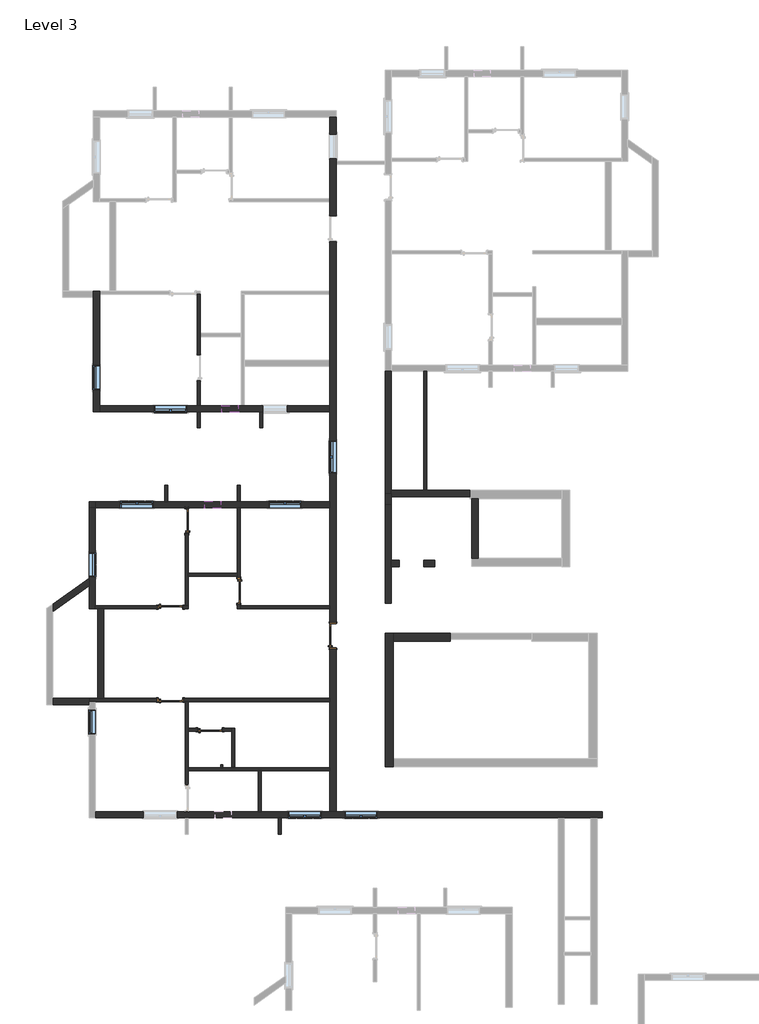
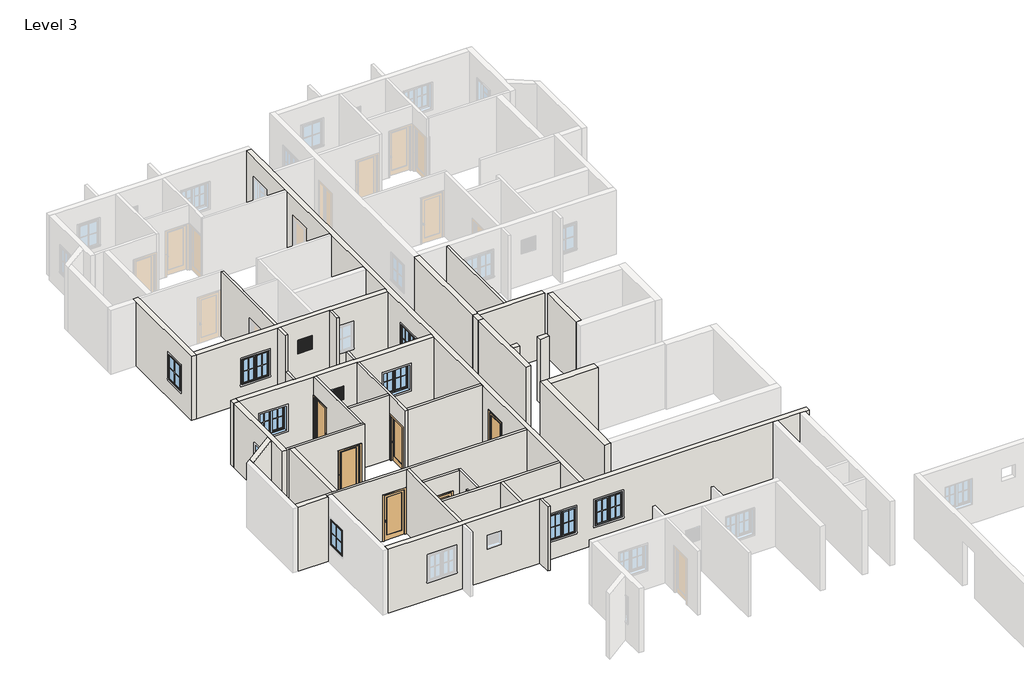
# One storey, part 4 of 7: 38 walls, 11 windows, 6 doors.
"""IFC4 building model written with IfcOpenShell, lengths in millimetres."""

from ifc_helpers import new_model, si_unit, frame, origin, place, context, project, spatial, polyline, outline, extrude, faceted_brep, transform, mapped, element, save
from components import door_a3feeac7, door_3c6ab76a, door_3b97b8e7, window_272f20d6, window_casement_double_4_x_4_af3140d2, window_f2d8fef0

model = new_model("IFC4")

# Units and contexts
model_context = context("Model", 3, world=origin())
ifc_project = project(units=[si_unit("LENGTHUNIT", "METRE", prefix="MILLI")], contexts=[model_context])

# Site, building, storey
site = spatial("IfcSite", under=ifc_project)
building = spatial("IfcBuilding", under=site)
storey = spatial("IfcBuildingStorey", under=building, Name="Level 3", Elevation=3200.4)

# Doors
placement = place(None, origin())
door_shape = door_a3feeac7(model_context)
element("IfcDoor", 1, ObjectType="Door-Interior-Single-1_Panel-Wood : 2'6\" x 7' door", at=placement, inside=storey, context=model_context, shape_type="MappedRepresentation", body=[
    mapped(door_shape, transform((-11252.4759469, 12427.2461172, 3200.4), x_axis=(0.0, 1.0, 0.0), y_axis=(-1.0, 0.0, 0.0), z_axis=(0.0, 0.0, 1.0))),
])
element("IfcDoor", 2, ObjectType="Door-Interior-Single-1_Panel-Wood : 2'6\" x 7' door", at=placement, inside=storey, context=model_context, shape_type="MappedRepresentation", body=[
    mapped(door_shape, transform((-10385.7009469, 4632.6211172, 3200.4), x_axis=(1.0, 0.0, 0.0), y_axis=(0.0, 1.0, 0.0), z_axis=(0.0, 0.0, 1.0))),
])
door_2_shape = door_3c6ab76a(model_context)
element("IfcDoor", 3, ObjectType="Door-Interior-Single-1_Panel-Wood : 36\" x 84\"", at=placement, inside=storey, context=model_context, shape_type="MappedRepresentation", body=[
    mapped(door_2_shape, transform((-9309.3759469, 9817.3961172, 3200.4), x_axis=(0.0, -1.0, 0.0), y_axis=(1.0, 0.0, 0.0), z_axis=(0.0, 0.0, 1.0))),
])
element("IfcDoor", 4, ObjectType="Door-Interior-Single-1_Panel-Wood : 36\" x 84\"", at=placement, inside=storey, context=model_context, shape_type="MappedRepresentation", body=[
    mapped(door_2_shape, transform((-11865.2509469, 9210.9711172, 3200.4), x_axis=(1.0, 0.0, 0.0), y_axis=(0.0, 1.0, 0.0), z_axis=(0.0, 0.0, 1.0))),
])
door_3_shape = door_3b97b8e7(model_context)
element("IfcDoor", 5, ObjectType="Door-Interior-Single-1_Panel-Wood : 36\" x 84\"", at=placement, inside=storey, context=model_context, shape_type="MappedRepresentation", body=[
    mapped(door_3_shape, transform((-5791.4759469, 8140.9961172, 3200.4), x_axis=(0.0, 1.0, 0.0), y_axis=(-1.0, 0.0, 0.0), z_axis=(0.0, 0.0, 1.0))),
])
element("IfcDoor", 6, ObjectType="Door-Interior-Single-1_Panel-Wood : 36\" x 84\"", at=placement, inside=storey, context=model_context, shape_type="MappedRepresentation", body=[
    mapped(door_shape, transform((-11865.2509469, 5737.5211172, 3200.4), x_axis=(1.0, 0.0, 0.0), y_axis=(0.0, 1.0, 0.0), z_axis=(0.0, 0.0, 1.0))),
])

# Walls
element("IfcWall", 7, ObjectType="1' feet", at=placement, inside=storey, context=model_context, shape_type="Brep", body=[
    faceted_brep([(-3540.4009469, 3245.1461172, 3200.4), (-3540.4009469, 3549.9461172, 3200.4), (-3540.4009469, 7931.4461172, 3200.4), (-3540.4009469, 8236.2461172, 3200.4), (-3540.4009469, 8236.2461172, 6248.4), (-3540.4009469, 7931.4461172, 6248.4), (-3540.4009469, 3549.9461172, 6248.4), (-3540.4009469, 3245.1461172, 6248.4), (-3845.2009469, 3245.1461172, 3200.4), (-3845.2009469, 3245.1461172, 6248.4), (-3845.2009469, 8236.2461172, 6248.4), (-3845.2009469, 8236.2461172, 3200.4)], [[[0, 1, 2, 3, 4, 5, 6, 7]], [[8, 9, 10, 11]], [[3, 2, 1, 0, 8, 11]], [[7, 6, 5, 4, 10, 9]], [[4, 3, 11, 10]], [[0, 7, 9, 8]]]),
])
element("IfcWall", 8, ObjectType="1' feet", at=placement, inside=storey, context=model_context, shape_type="Brep", body=[
    faceted_brep([(-3540.4009469, 7931.4461172, 3200.4), (-1406.8009469, 7931.4461172, 3200.4), (-1406.8009469, 7931.4461172, 6248.4), (-3540.4009469, 7931.4461172, 6248.4), (-3540.4009469, 8236.2461172, 3200.4), (-3540.4009469, 8236.2461172, 6248.4), (-1406.8009469, 8236.2461172, 6248.4), (-1406.8009469, 8236.2461172, 3200.4), (-1406.8009469, 8007.6461172, 3200.4), (-1406.8009469, 8007.6461172, 6248.4)], [[[0, 1, 2, 3]], [[4, 5, 6, 7]], [[1, 0, 4, 7, 8]], [[2, 1, 8, 7, 6, 9]], [[3, 2, 9, 6, 5]], [[0, 3, 5, 4]]]),
])
element("IfcWall", 9, ObjectType="4.5\" wall", at=placement, inside=storey, context=model_context, shape_type="Brep", body=[
    faceted_brep([(-10741.3009469, 20898.1461172, 6248.4), (-10741.3009469, 19437.6461172, 6248.4), (-10741.3009469, 19323.3461172, 6248.4), (-10741.3009469, 16732.5461172, 6248.4), (-10741.3009469, 16732.5461172, 3200.4), (-10741.3009469, 17678.6961172, 3200.4), (-10741.3009469, 17678.6961172, 5359.4), (-10741.3009469, 18643.8961172, 5359.4), (-10741.3009469, 18643.8961172, 3200.4), (-10741.3009469, 19323.3461172, 3200.4), (-10741.3009469, 19437.6461172, 3200.4), (-10741.3009469, 20898.1461172, 3200.4), (-10855.6009469, 16732.5461172, 6248.4), (-10855.6009469, 20898.1461172, 6248.4), (-10855.6009469, 20898.1461172, 3200.4), (-10855.6009469, 18643.8961172, 3200.4), (-10855.6009469, 18643.8961172, 5359.4), (-10855.6009469, 17678.6961172, 5359.4), (-10855.6009469, 17678.6961172, 3200.4), (-10855.6009469, 16732.5461172, 3200.4)], [[[0, 1, 2, 3, 4, 5, 6, 7, 8, 9, 10, 11]], [[12, 13, 14, 15, 16, 17, 18, 19]], [[4, 19, 18, 5]], [[14, 11, 10, 9, 8, 15]], [[3, 2, 1, 0, 13, 12]], [[4, 3, 12, 19]], [[0, 11, 14, 13]], [[7, 16, 15, 8]], [[16, 7, 6, 17]], [[17, 6, 5, 18]]]),
])
element("IfcWall", 10, ObjectType="4.5\" wall", at=placement, inside=storey, context=model_context, shape_type="Brep", body=[
    faceted_brep([(-9369.7009469, 9150.6461172, 6248.4), (-9369.7009469, 10369.8461172, 6248.4), (-9369.7009469, 10484.1461172, 6248.4), (-9369.7009469, 12922.5461172, 6248.4), (-9369.7009469, 12922.5461172, 3200.4), (-9369.7009469, 10484.1461172, 3200.4), (-9369.7009469, 10369.8461172, 3200.4), (-9369.7009469, 10299.9961172, 3200.4), (-9369.7009469, 10299.9961172, 5359.4), (-9369.7009469, 9334.7961172, 5359.4), (-9369.7009469, 9334.7961172, 3200.4), (-9369.7009469, 9150.6461172, 3200.4), (-9255.4009469, 12922.5461172, 6248.4), (-9255.4009469, 9264.9461172, 6248.4), (-9255.4009469, 9150.6461172, 6248.4), (-9255.4009469, 9150.6461172, 3200.4), (-9255.4009469, 9264.9461172, 3200.4), (-9255.4009469, 9334.7961172, 3200.4), (-9255.4009469, 9334.7961172, 5359.4), (-9255.4009469, 10299.9961172, 5359.4), (-9255.4009469, 10299.9961172, 3200.4), (-9255.4009469, 12922.5461172, 3200.4)], [[[0, 1, 2, 3, 4, 5, 6, 7, 8, 9, 10, 11]], [[12, 13, 14, 15, 16, 17, 18, 19, 20, 21]], [[4, 21, 20, 7, 6, 5]], [[15, 11, 10, 17, 16]], [[3, 2, 1, 0, 14, 13, 12]], [[4, 3, 12, 21]], [[0, 11, 15, 14]], [[9, 18, 17, 10]], [[18, 9, 8, 19]], [[19, 8, 7, 20]]]),
])
element("IfcWall", 11, ObjectType="4.5\" wall", at=placement, inside=storey, context=model_context, shape_type="SweptSolid", body=[
    extrude(outline(polyline([(-11198.5009469, 10484.1461172), (-9369.7009469, 10484.1461172), (-9369.7009469, 10369.8461172), (-11198.5009469, 10369.8461172), (-11198.5009469, 10484.1461172)])), frame((0.0, 0.0, 3200.4), z_axis=(0.0, 0.0, 1.0), x_axis=(1.0, 0.0, 0.0)), (0.0, 0.0, 1.0), 3048.0),
])
element("IfcWall", 12, ObjectType="4.5\" wall", at=placement, inside=storey, context=model_context, shape_type="Brep", body=[
    faceted_brep([(-11312.8009469, 9264.9461172, 6248.4), (-11312.8009469, 12922.5461172, 6248.4), (-11312.8009469, 12922.5461172, 3200.4), (-11312.8009469, 12909.8461172, 3200.4), (-11312.8009469, 12909.8461172, 5359.4), (-11312.8009469, 11944.6461172, 5359.4), (-11312.8009469, 11944.6461172, 3200.4), (-11312.8009469, 9264.9461172, 3200.4), (-11198.5009469, 12922.5461172, 6248.4), (-11198.5009469, 10484.1461172, 6248.4), (-11198.5009469, 10369.8461172, 6248.4), (-11198.5009469, 9264.9461172, 6248.4), (-11198.5009469, 9264.9461172, 3200.4), (-11198.5009469, 10369.8461172, 3200.4), (-11198.5009469, 10484.1461172, 3200.4), (-11198.5009469, 11944.6461172, 3200.4), (-11198.5009469, 11944.6461172, 5359.4), (-11198.5009469, 12909.8461172, 5359.4), (-11198.5009469, 12909.8461172, 3200.4), (-11198.5009469, 12922.5461172, 3200.4)], [[[0, 1, 2, 3, 4, 5, 6, 7]], [[8, 9, 10, 11, 12, 13, 14, 15, 16, 17, 18, 19]], [[12, 7, 6, 15, 14, 13]], [[2, 19, 18, 3]], [[1, 0, 11, 10, 9, 8]], [[0, 7, 12, 11]], [[2, 1, 8, 19]], [[17, 4, 3, 18]], [[4, 17, 16, 5]], [[5, 16, 15, 6]]]),
])
element("IfcWall", 13, ObjectType="4.5\" wall", at=placement, inside=storey, context=model_context, shape_type="Brep", body=[
    faceted_brep([(-14665.6009469, 9264.9461172, 6248.4), (-11312.8009469, 9264.9461172, 6248.4), (-11198.5009469, 9264.9461172, 6248.4), (-11198.5009469, 9264.9461172, 3200.4), (-11312.8009469, 9264.9461172, 3200.4), (-11382.6509469, 9264.9461172, 3200.4), (-11382.6509469, 9264.9461172, 5359.4), (-12347.8509469, 9264.9461172, 5359.4), (-12347.8509469, 9264.9461172, 3200.4), (-14665.6009469, 9264.9461172, 3200.4), (-11198.5009469, 9150.6461172, 6248.4), (-14360.8009469, 9150.6461172, 6248.4), (-14589.4009469, 9150.6461172, 6248.4), (-14665.6009469, 9150.6461172, 6248.4), (-14665.6009469, 9150.6461172, 3200.4), (-14589.4009469, 9150.6461172, 3200.4), (-14360.8009469, 9150.6461172, 3200.4), (-12347.8509469, 9150.6461172, 3200.4), (-12347.8509469, 9150.6461172, 5359.4), (-11382.6509469, 9150.6461172, 5359.4), (-11382.6509469, 9150.6461172, 3200.4), (-11198.5009469, 9150.6461172, 3200.4)], [[[0, 1, 2, 3, 4, 5, 6, 7, 8, 9]], [[10, 11, 12, 13, 14, 15, 16, 17, 18, 19, 20, 21]], [[3, 21, 20, 5, 4]], [[14, 9, 8, 17, 16, 15]], [[2, 1, 0, 13, 12, 11, 10]], [[3, 2, 10, 21]], [[0, 9, 14, 13]], [[19, 6, 5, 20]], [[6, 19, 18, 7]], [[7, 18, 17, 8]]]),
])
element("IfcWall", 14, ObjectType="4.5\" wall", at=placement, inside=storey, context=model_context, shape_type="SweptSolid", body=[
    extrude(outline(polyline([(-9255.4009469, 9264.9461172), (-5902.6009469, 9264.9461172), (-5902.6009469, 9150.6461172), (-9255.4009469, 9150.6461172), (-9255.4009469, 9264.9461172)])), frame((0.0, 0.0, 3200.4), z_axis=(0.0, 0.0, 1.0), x_axis=(1.0, 0.0, 0.0)), (0.0, 0.0, 1.0), 3048.0),
])
element("IfcWall", 15, ObjectType="4.5\" wall", at=placement, inside=storey, context=model_context, shape_type="Brep", body=[
    faceted_brep([(-5902.6009469, 5683.5461172, 6248.4), (-11198.5009469, 5683.5461172, 6248.4), (-11312.8009469, 5683.5461172, 6248.4), (-14665.6009469, 5683.5461172, 6248.4), (-14894.2009469, 5683.5461172, 6248.4), (-14894.2009469, 5683.5461172, 3200.4), (-14665.6009469, 5683.5461172, 3200.4), (-12347.8509469, 5683.5461172, 3200.4), (-12347.8509469, 5683.5461172, 5359.4), (-11382.6509469, 5683.5461172, 5359.4), (-11382.6509469, 5683.5461172, 3200.4), (-11312.8009469, 5683.5461172, 3200.4), (-11198.5009469, 5683.5461172, 3200.4), (-5902.6009469, 5683.5461172, 3200.4), (-14894.2009469, 5797.8461172, 6248.4), (-14589.4009469, 5797.8461172, 6248.4), (-14360.8009469, 5797.8461172, 6248.4), (-5902.6009469, 5797.8461172, 6248.4), (-5902.6009469, 5797.8461172, 3200.4), (-11382.6509469, 5797.8461172, 3200.4), (-11382.6509469, 5797.8461172, 5359.4), (-12347.8509469, 5797.8461172, 5359.4), (-12347.8509469, 5797.8461172, 3200.4), (-14360.8009469, 5797.8461172, 3200.4), (-14589.4009469, 5797.8461172, 3200.4), (-14894.2009469, 5797.8461172, 3200.4)], [[[0, 1, 2, 3, 4, 5, 6, 7, 8, 9, 10, 11, 12, 13]], [[14, 15, 16, 17, 18, 19, 20, 21, 22, 23, 24, 25]], [[18, 13, 12, 11, 10, 19]], [[5, 25, 24, 23, 22, 7, 6]], [[4, 3, 2, 1, 0, 17, 16, 15, 14]], [[0, 13, 18, 17]], [[5, 4, 14, 25]], [[9, 20, 19, 10]], [[20, 9, 8, 21]], [[21, 8, 7, 22]]]),
])
element("IfcWall", 16, ObjectType="4.5\" wall", at=placement, inside=storey, context=model_context, shape_type="Brep", body=[
    faceted_brep([(-11198.5009469, 5683.5461172, 6248.4), (-11198.5009469, 4692.9461172, 6248.4), (-11198.5009469, 4578.6461172, 6248.4), (-11198.5009469, 3207.0461172, 6248.4), (-11198.5009469, 3092.7461172, 6248.4), (-11198.5009469, 1568.7461172, 6248.4), (-11198.5009469, 1568.7461172, 3200.4), (-11198.5009469, 1581.4461172, 3200.4), (-11198.5009469, 1581.4461172, 5359.4), (-11198.5009469, 2546.6461172, 5359.4), (-11198.5009469, 2546.6461172, 3200.4), (-11198.5009469, 3092.7461172, 3200.4), (-11198.5009469, 3207.0461172, 3200.4), (-11198.5009469, 4578.6461172, 3200.4), (-11198.5009469, 4692.9461172, 3200.4), (-11198.5009469, 5683.5461172, 3200.4), (-11312.8009469, 1568.7461172, 6248.4), (-11312.8009469, 5683.5461172, 6248.4), (-11312.8009469, 5683.5461172, 3200.4), (-11312.8009469, 2546.6461172, 3200.4), (-11312.8009469, 2546.6461172, 5359.4), (-11312.8009469, 1581.4461172, 5359.4), (-11312.8009469, 1581.4461172, 3200.4), (-11312.8009469, 1568.7461172, 3200.4)], [[[0, 1, 2, 3, 4, 5, 6, 7, 8, 9, 10, 11, 12, 13, 14, 15]], [[16, 17, 18, 19, 20, 21, 22, 23]], [[18, 15, 14, 13, 12, 11, 10, 19]], [[6, 23, 22, 7]], [[5, 4, 3, 2, 1, 0, 17, 16]], [[0, 15, 18, 17]], [[6, 5, 16, 23]], [[21, 8, 7, 22]], [[8, 21, 20, 9]], [[9, 20, 19, 10]]]),
])
element("IfcWall", 17, ObjectType="4.5\" wall", at=placement, inside=storey, context=model_context, shape_type="SweptSolid", body=[
    extrude(outline(polyline([(-9985.226836, 3326.5226372), (-9915.376836, 3326.5226372), (-9915.376836, 3212.2226372), (-9985.226836, 3212.2226372), (-9985.226836, 3326.5226372)])), frame((0.0, 0.0, 3200.4), z_axis=(0.0, 0.0, 1.0), x_axis=(1.0, 0.0, 0.0)), (0.0, 0.0, 1.0), 3048.0),
])
element("IfcWall", 18, ObjectType="4.5\" wall", at=placement, inside=storey, context=model_context, shape_type="Brep", body=[
    faceted_brep([(-5902.6009469, 3207.0461172, 3200.4), (-11198.5009469, 3207.0461172, 3200.4), (-11198.5009469, 3207.0461172, 6248.4), (-5902.6009469, 3207.0461172, 6248.4), (-5902.6009469, 3092.7461172, 3200.4), (-5902.6009469, 3092.7461172, 6248.4), (-8468.0009469, 3092.7461172, 6248.4), (-8582.3009469, 3092.7461172, 6248.4), (-11198.5009469, 3092.7461172, 6248.4), (-11198.5009469, 3092.7461172, 3200.4), (-8582.3009469, 3092.7461172, 3200.4), (-8468.0009469, 3092.7461172, 3200.4)], [[[0, 1, 2, 3]], [[4, 5, 6, 7, 8, 9, 10, 11]], [[1, 0, 4, 11, 10, 9]], [[3, 2, 8, 7, 6, 5]], [[2, 1, 9, 8]], [[0, 3, 5, 4]]]),
])
element("IfcWall", 19, ObjectType="4.5\" wall", at=placement, inside=storey, context=model_context, shape_type="SweptSolid", body=[
    extrude(outline(polyline([(-8582.3009469, 1568.7461172), (-8582.3009469, 3092.7461172), (-8468.0009469, 3092.7461172), (-8468.0009469, 1568.7461172), (-8582.3009469, 1568.7461172)])), frame((0.0, 0.0, 3200.4), z_axis=(0.0, 0.0, 1.0), x_axis=(1.0, 0.0, 0.0)), (0.0, 0.0, 1.0), 3048.0),
])
element("IfcWall", 20, ObjectType="4.5\" wall", at=placement, inside=storey, context=model_context, shape_type="Brep", body=[
    faceted_brep([(-9572.9009469, 4692.9461172, 3200.4), (-9572.9009469, 4578.6461172, 3200.4), (-9572.9009469, 3245.1461172, 3200.4), (-9572.9009469, 3245.1461172, 6248.4), (-9572.9009469, 4578.6461172, 6248.4), (-9572.9009469, 4692.9461172, 6248.4), (-9458.6009469, 4692.9461172, 3200.4), (-9458.6009469, 4692.9461172, 6248.4), (-9458.6009469, 3245.1461172, 6248.4), (-9458.6009469, 3245.1461172, 3200.4)], [[[0, 1, 2, 3, 4, 5]], [[6, 7, 8, 9]], [[2, 1, 0, 6, 9]], [[3, 2, 9, 8]], [[5, 4, 3, 8, 7]], [[0, 5, 7, 6]]]),
])
element("IfcWall", 21, ObjectType="4.5\" wall", at=placement, inside=storey, context=model_context, shape_type="SweptSolid", body=[
    extrude(outline(polyline([(6248.4, -9572.9009469), (6248.4, -11198.5009469), (3200.4, -11198.5009469), (3200.4, -10868.3009469), (5359.4, -10868.3009469), (5359.4, -9903.1009469), (3200.4, -9903.1009469), (3200.4, -9572.9009469), (6248.4, -9572.9009469)])), frame((0.0, 4578.6461172, 0.0), z_axis=(0.0, 1.0, 0.0), x_axis=(0.0, 0.0, 1.0)), (0.0, 0.0, 1.0), 114.3),
])
element("IfcWall", 22, ObjectType="4.5\" wall", at=placement, inside=storey, context=model_context, shape_type="SweptSolid", body=[
    extrude(outline(polyline([(-7841.0333092, 730.5461172), (-7841.0333092, 1340.1461172), (-7726.7333092, 1340.1461172), (-7726.7333092, 730.5461172), (-7841.0333092, 730.5461172)])), frame((0.0, 0.0, 3200.4), z_axis=(0.0, 0.0, 1.0), x_axis=(1.0, 0.0, 0.0)), (0.0, 0.0, 1.0), 3048.0),
])
element("IfcWall", 23, ObjectType="4.5\" wall", at=placement, inside=storey, context=model_context, shape_type="SweptSolid", body=[
    extrude(outline(polyline([(-10855.6009469, 15918.3895495), (-10855.6009469, 16503.9461172), (-10741.3009469, 16503.9461172), (-10741.3009469, 15918.3895495), (-10855.6009469, 15918.3895495)])), frame((0.0, 0.0, 3200.4), z_axis=(0.0, 0.0, 1.0), x_axis=(1.0, 0.0, 0.0)), (0.0, 0.0, 1.0), 3048.0),
])
element("IfcWall", 24, ObjectType="4.5\" wall", at=placement, inside=storey, context=model_context, shape_type="Brep", body=[
    faceted_brep([(-8531.5009469, 16503.9461172, 3200.4), (-8531.5009469, 15918.3895495, 3200.4), (-8531.5009469, 15918.3895495, 6248.4), (-8531.5009469, 16503.9461172, 6248.4), (-8417.2009469, 16503.9461172, 3200.4), (-8417.2009469, 16503.9461172, 4114.8), (-8417.2009469, 16503.9461172, 5334.0), (-8417.2009469, 16503.9461172, 6248.4), (-8417.2009469, 15918.3895495, 6248.4), (-8417.2009469, 15918.3895495, 3200.4)], [[[0, 1, 2, 3]], [[4, 5, 6, 7, 8, 9]], [[1, 0, 4, 9]], [[2, 1, 9, 8]], [[3, 2, 8, 7]], [[0, 3, 7, 6, 5, 4]]]),
])
element("IfcWall", 25, ObjectType="4.5\" wall", at=placement, inside=storey, context=model_context, shape_type="SweptSolid", body=[
    extrude(outline(polyline([(-12085.9698258, 13151.1461172), (-12085.9698258, 13760.7461172), (-11971.6698258, 13760.7461172), (-11971.6698258, 13151.1461172), (-12085.9698258, 13151.1461172)])), frame((0.0, 0.0, 3200.4), z_axis=(0.0, 0.0, 1.0), x_axis=(1.0, 0.0, 0.0)), (0.0, 0.0, 1.0), 3048.0),
])
element("IfcWall", 26, ObjectType="4.5\" wall", at=placement, inside=storey, context=model_context, shape_type="SweptSolid", body=[
    extrude(outline(polyline([(-9255.4009469, 13760.7461172), (-9255.4009469, 13151.1461172), (-9369.7009469, 13151.1461172), (-9369.7009469, 13760.7461172), (-9255.4009469, 13760.7461172)])), frame((0.0, 0.0, 3200.4), z_axis=(0.0, 0.0, 1.0), x_axis=(1.0, 0.0, 0.0)), (0.0, 0.0, 1.0), 3048.0),
])
element("IfcWall", 27, ObjectType="4.5\" wall", at=placement, inside=storey, context=model_context, shape_type="SweptSolid", body=[
    extrude(outline(polyline([(-2402.381873, 13571.4182723), (-2402.381873, 18017.4255084), (-2288.081873, 18017.4255084), (-2288.081873, 13571.4182723), (-2402.381873, 13571.4182723)])), frame((0.0, 0.0, 3200.4), z_axis=(0.0, 0.0, 1.0), x_axis=(1.0, 0.0, 0.0)), (0.0, 0.0, 1.0), 3048.0),
])
element("IfcWall", 28, ObjectType="9\"", at=placement, inside=storey, context=model_context, shape_type="Brep", body=[
    faceted_brep([(-14513.2009469, 16503.9461172, 3200.4), (-14513.2009469, 16732.5461172, 3200.4), (-14513.2009469, 20898.1461172, 3200.4), (-14513.2009469, 21012.4461172, 3200.4), (-14513.2009469, 21012.4461172, 6248.4), (-14513.2009469, 20898.1461172, 6248.4), (-14513.2009469, 16732.5461172, 6248.4), (-14513.2009469, 16503.9461172, 6248.4), (-14513.2009469, 18243.8461172, 5334.0), (-14513.2009469, 18243.8461172, 4114.8), (-14513.2009469, 17329.4461172, 4114.8), (-14513.2009469, 17329.4461172, 5334.0), (-14741.8009469, 16503.9461172, 3200.4), (-14741.8009469, 16503.9461172, 6248.4), (-14741.8009469, 20783.8461172, 6248.4), (-14741.8009469, 21012.4461172, 6248.4), (-14741.8009469, 21012.4461172, 3200.4), (-14741.8009469, 20783.8461172, 3200.4), (-14741.8009469, 18243.8461172, 5334.0), (-14741.8009469, 17329.4461172, 5334.0), (-14741.8009469, 17329.4461172, 4114.8), (-14741.8009469, 18243.8461172, 4114.8)], [[[0, 1, 2, 3, 4, 5, 6, 7], [8, 9, 10, 11]], [[12, 13, 14, 15, 16, 17], [18, 19, 20, 21]], [[3, 2, 1, 0, 12, 17, 16]], [[7, 6, 5, 4, 15, 14, 13]], [[4, 3, 16, 15]], [[0, 7, 13, 12]], [[9, 8, 18, 21]], [[10, 9, 21, 20]], [[11, 10, 20, 19]], [[8, 11, 19, 18]]]),
])
element("IfcWall", 29, ObjectType="9\"", at=placement, inside=storey, context=model_context, shape_type="Brep", body=[
    faceted_brep([(-5902.6009469, 1568.7461172, 6248.4), (-5902.6009469, 3092.7461172, 6248.4), (-5902.6009469, 3207.0461172, 6248.4), (-5902.6009469, 5683.5461172, 6248.4), (-5902.6009469, 5797.8461172, 6248.4), (-5902.6009469, 9150.6461172, 6248.4), (-5902.6009469, 9264.9461172, 6248.4), (-5902.6009469, 12922.5461172, 6248.4), (-5902.6009469, 13151.1461172, 6248.4), (-5902.6009469, 16503.9461172, 6248.4), (-5902.6009469, 16732.5461172, 6248.4), (-5902.6009469, 18205.7461172, 6248.4), (-5902.6009469, 18434.3461172, 6248.4), (-5902.6009469, 20898.1461172, 6248.4), (-5902.6009469, 21012.4461172, 6248.4), (-5902.6009469, 24365.2461172, 6248.4), (-5902.6009469, 24479.5461172, 6248.4), (-5902.6009469, 27527.5461172, 6248.4), (-5902.6009469, 27527.5461172, 3200.4), (-5902.6009469, 24479.5461172, 3200.4), (-5902.6009469, 24365.2461172, 3200.4), (-5902.6009469, 23838.1961172, 3200.4), (-5902.6009469, 23838.1961172, 5359.4), (-5902.6009469, 22872.9961172, 5359.4), (-5902.6009469, 22872.9961172, 3200.4), (-5902.6009469, 21012.4461172, 3200.4), (-5902.6009469, 20898.1461172, 3200.4), (-5902.6009469, 18434.3461172, 3200.4), (-5902.6009469, 18205.7461172, 3200.4), (-5902.6009469, 16732.5461172, 3200.4), (-5902.6009469, 16503.9461172, 3200.4), (-5902.6009469, 13151.1461172, 3200.4), (-5902.6009469, 12922.5461172, 3200.4), (-5902.6009469, 9264.9461172, 3200.4), (-5902.6009469, 9150.6461172, 3200.4), (-5902.6009469, 8623.5961172, 3200.4), (-5902.6009469, 8623.5961172, 5359.4), (-5902.6009469, 7658.3961172, 5359.4), (-5902.6009469, 7658.3961172, 3200.4), (-5902.6009469, 5797.8461172, 3200.4), (-5902.6009469, 5683.5461172, 3200.4), (-5902.6009469, 3207.0461172, 3200.4), (-5902.6009469, 3092.7461172, 3200.4), (-5902.6009469, 1568.7461172, 3200.4), (-5902.6009469, 25973.9755084, 5334.0), (-5902.6009469, 25973.9755084, 4114.8), (-5902.6009469, 26888.3755084, 4114.8), (-5902.6009469, 26888.3755084, 5334.0), (-5902.6009469, 15437.1461172, 5334.0), (-5902.6009469, 14217.9461172, 5334.0), (-5902.6009469, 14217.9461172, 4114.8), (-5902.6009469, 15437.1461172, 4114.8), (-5674.0009469, 27527.5461172, 6248.4), (-5674.0009469, 25878.7255084, 6248.4), (-5674.0009469, 25764.4255084, 6248.4), (-5674.0009469, 1568.7461172, 6248.4), (-5674.0009469, 1568.7461172, 3200.4), (-5674.0009469, 7658.3961172, 3200.4), (-5674.0009469, 7658.3961172, 5359.4), (-5674.0009469, 8623.5961172, 5359.4), (-5674.0009469, 8623.5961172, 3200.4), (-5674.0009469, 22872.9961172, 3200.4), (-5674.0009469, 22872.9961172, 5359.4), (-5674.0009469, 23838.1961172, 5359.4), (-5674.0009469, 23838.1961172, 3200.4), (-5674.0009469, 25764.4255084, 3200.4), (-5674.0009469, 25878.7255084, 3200.4), (-5674.0009469, 27527.5461172, 3200.4), (-5674.0009469, 27527.5461172, 3352.8), (-5674.0009469, 25973.9755084, 5334.0), (-5674.0009469, 26888.3755084, 5334.0), (-5674.0009469, 26888.3755084, 4114.8), (-5674.0009469, 25973.9755084, 4114.8), (-5674.0009469, 15437.1461172, 5334.0), (-5674.0009469, 15437.1461172, 4114.8), (-5674.0009469, 14217.9461172, 4114.8), (-5674.0009469, 14217.9461172, 5334.0)], [[[0, 1, 2, 3, 4, 5, 6, 7, 8, 9, 10, 11, 12, 13, 14, 15, 16, 17, 18, 19, 20, 21, 22, 23, 24, 25, 26, 27, 28, 29, 30, 31, 32, 33, 34, 35, 36, 37, 38, 39, 40, 41, 42, 43], [44, 45, 46, 47], [48, 49, 50, 51]], [[52, 53, 54, 55, 56, 57, 58, 59, 60, 61, 62, 63, 64, 65, 66, 67, 68], [69, 70, 71, 72], [73, 74, 75, 76]], [[18, 67, 66, 65, 64, 21, 20, 19]], [[56, 43, 42, 41, 40, 39, 38, 57]], [[24, 61, 60, 35, 34, 33, 32, 31, 30, 29, 28, 27, 26, 25]], [[17, 16, 15, 14, 13, 12, 11, 10, 9, 8, 7, 6, 5, 4, 3, 2, 1, 0, 55, 54, 53, 52]], [[18, 17, 52, 68, 67]], [[0, 43, 56, 55]], [[63, 22, 21, 64]], [[22, 63, 62, 23]], [[23, 62, 61, 24]], [[59, 36, 35, 60]], [[36, 59, 58, 37]], [[37, 58, 57, 38]], [[45, 44, 69, 72]], [[46, 45, 72, 71]], [[47, 46, 71, 70]], [[44, 47, 70, 69]], [[74, 73, 48, 51]], [[75, 74, 51, 50]], [[76, 75, 50, 49]], [[73, 76, 49, 48]]]),
])
element("IfcWall", 30, ObjectType="9\"", at=placement, inside=storey, context=model_context, shape_type="Brep", body=[
    faceted_brep([(-14513.2009469, 16503.9461172, 3200.4), (-10855.6009469, 16503.9461172, 3200.4), (-10741.3009469, 16503.9461172, 3200.4), (-8531.5009469, 16503.9461172, 3200.4), (-8417.2009469, 16503.9461172, 3200.4), (-5902.6009469, 16503.9461172, 3200.4), (-5902.6009469, 16503.9461172, 6248.4), (-8417.2009469, 16503.9461172, 6248.4), (-8531.5009469, 16503.9461172, 6248.4), (-10741.3009469, 16503.9461172, 6248.4), (-10855.6009469, 16503.9461172, 6248.4), (-14513.2009469, 16503.9461172, 6248.4), (-9337.9509469, 16503.9461172, 5334.0), (-9337.9509469, 16503.9461172, 4724.4), (-9947.5509469, 16503.9461172, 4724.4), (-9947.5509469, 16503.9461172, 5334.0), (-8417.2009469, 16503.9461172, 5334.0), (-7502.8009469, 16503.9461172, 5334.0), (-7502.8009469, 16503.9461172, 4114.8), (-8417.2009469, 16503.9461172, 4114.8), (-12474.8509469, 16503.9461172, 5334.0), (-11255.6509469, 16503.9461172, 5334.0), (-11255.6509469, 16503.9461172, 4114.8), (-12474.8509469, 16503.9461172, 4114.8), (-14513.2009469, 16732.5461172, 3200.4), (-14513.2009469, 16732.5461172, 6248.4), (-10855.6009469, 16732.5461172, 6248.4), (-10741.3009469, 16732.5461172, 6248.4), (-9217.3009469, 16732.5461172, 6248.4), (-9103.0009469, 16732.5461172, 6248.4), (-5902.6009469, 16732.5461172, 6248.4), (-5902.6009469, 16732.5461172, 3200.4), (-9103.0009469, 16732.5461172, 3200.4), (-9217.3009469, 16732.5461172, 3200.4), (-10741.3009469, 16732.5461172, 3200.4), (-10855.6009469, 16732.5461172, 3200.4), (-9337.9509469, 16732.5461172, 5334.0), (-9947.5509469, 16732.5461172, 5334.0), (-9947.5509469, 16732.5461172, 4724.4), (-9337.9509469, 16732.5461172, 4724.4), (-8417.2009469, 16732.5461172, 5334.0), (-8417.2009469, 16732.5461172, 4114.8), (-7502.8009469, 16732.5461172, 4114.8), (-7502.8009469, 16732.5461172, 5334.0), (-12474.8509469, 16732.5461172, 5334.0), (-12474.8509469, 16732.5461172, 4114.8), (-11255.6509469, 16732.5461172, 4114.8), (-11255.6509469, 16732.5461172, 5334.0)], [[[0, 1, 2, 3, 4, 5, 6, 7, 8, 9, 10, 11], [12, 13, 14, 15], [16, 17, 18, 19], [20, 21, 22, 23]], [[24, 25, 26, 27, 28, 29, 30, 31, 32, 33, 34, 35], [36, 37, 38, 39], [40, 41, 42, 43], [44, 45, 46, 47]], [[5, 4, 3, 2, 1, 0, 24, 35, 34, 33, 32, 31]], [[11, 10, 9, 8, 7, 6, 30, 29, 28, 27, 26, 25]], [[6, 5, 31, 30]], [[0, 11, 25, 24]], [[13, 12, 36, 39]], [[14, 13, 39, 38]], [[15, 14, 38, 37]], [[12, 15, 37, 36]], [[41, 40, 16, 19]], [[42, 41, 19, 18]], [[43, 42, 18, 17]], [[40, 43, 17, 16]], [[45, 44, 20, 23]], [[46, 45, 23, 22]], [[47, 46, 22, 21]], [[44, 47, 21, 20]]]),
])
element("IfcWall", 31, ObjectType="9\"", at=placement, inside=storey, context=model_context, shape_type="Brep", body=[
    faceted_brep([(-5902.6009469, 13151.1461172, 3200.4), (-9255.4009469, 13151.1461172, 3200.4), (-9369.7009469, 13151.1461172, 3200.4), (-11971.6698258, 13151.1461172, 3200.4), (-12085.9698258, 13151.1461172, 3200.4), (-14665.6009469, 13151.1461172, 3200.4), (-14665.6009469, 13151.1461172, 6248.4), (-12085.9698258, 13151.1461172, 6248.4), (-11971.6698258, 13151.1461172, 6248.4), (-9369.7009469, 13151.1461172, 6248.4), (-9255.4009469, 13151.1461172, 6248.4), (-5902.6009469, 13151.1461172, 6248.4), (-9979.3009469, 13151.1461172, 5334.0), (-10588.9009469, 13151.1461172, 5334.0), (-10588.9009469, 13151.1461172, 4724.4), (-9979.3009469, 13151.1461172, 4724.4), (-12511.4198258, 13151.1461172, 5334.0), (-13730.6198258, 13151.1461172, 5334.0), (-13730.6198258, 13151.1461172, 4114.8), (-12511.4198258, 13151.1461172, 4114.8), (-6975.7509469, 13151.1461172, 5334.0), (-8194.9509469, 13151.1461172, 5334.0), (-8194.9509469, 13151.1461172, 4114.8), (-6975.7509469, 13151.1461172, 4114.8), (-5902.6009469, 12922.5461172, 3200.4), (-5902.6009469, 12922.5461172, 6248.4), (-9255.4009469, 12922.5461172, 6248.4), (-9369.7009469, 12922.5461172, 6248.4), (-11198.5009469, 12922.5461172, 6248.4), (-11312.8009469, 12922.5461172, 6248.4), (-14665.6009469, 12922.5461172, 6248.4), (-14665.6009469, 12922.5461172, 3200.4), (-11312.8009469, 12922.5461172, 3200.4), (-11198.5009469, 12922.5461172, 3200.4), (-9369.7009469, 12922.5461172, 3200.4), (-9255.4009469, 12922.5461172, 3200.4), (-9979.3009469, 12922.5461172, 5334.0), (-9979.3009469, 12922.5461172, 4724.4), (-10588.9009469, 12922.5461172, 4724.4), (-10588.9009469, 12922.5461172, 5334.0), (-12511.4198258, 12922.5461172, 5334.0), (-12511.4198258, 12922.5461172, 4114.8), (-13730.6198258, 12922.5461172, 4114.8), (-13730.6198258, 12922.5461172, 5334.0), (-6975.7509469, 12922.5461172, 5334.0), (-6975.7509469, 12922.5461172, 4114.8), (-8194.9509469, 12922.5461172, 4114.8), (-8194.9509469, 12922.5461172, 5334.0)], [[[0, 1, 2, 3, 4, 5, 6, 7, 8, 9, 10, 11], [12, 13, 14, 15], [16, 17, 18, 19], [20, 21, 22, 23]], [[24, 25, 26, 27, 28, 29, 30, 31, 32, 33, 34, 35], [36, 37, 38, 39], [40, 41, 42, 43], [44, 45, 46, 47]], [[5, 4, 3, 2, 1, 0, 24, 35, 34, 33, 32, 31]], [[11, 10, 9, 8, 7, 6, 30, 29, 28, 27, 26, 25]], [[6, 5, 31, 30]], [[0, 11, 25, 24]], [[37, 36, 12, 15]], [[38, 37, 15, 14]], [[39, 38, 14, 13]], [[36, 39, 13, 12]], [[41, 40, 16, 19]], [[42, 41, 19, 18]], [[43, 42, 18, 17]], [[40, 43, 17, 16]], [[45, 44, 20, 23]], [[46, 45, 23, 22]], [[47, 46, 22, 21]], [[44, 47, 21, 20]]]),
])
element("IfcWall", 32, ObjectType="9\"", at=placement, inside=storey, context=model_context, shape_type="SweptSolid", body=[
    extrude(outline(polyline([(-14894.2009469, 12922.5461172), (-14894.2009469, 13151.1461172), (-14665.6009469, 13151.1461172), (-14665.6009469, 12922.5461172), (-14894.2009469, 12922.5461172)])), frame((0.0, 0.0, 3200.4), z_axis=(0.0, 0.0, 1.0), x_axis=(1.0, 0.0, 0.0)), (0.0, 0.0, 1.0), 3048.0),
])
element("IfcWall", 33, ObjectType="9\"", at=placement, inside=storey, context=model_context, shape_type="SweptSolid", body=[
    extrude(outline(polyline([(-14589.4009469, 5797.8461172), (-14589.4009469, 9150.6461172), (-14360.8009469, 9150.6461172), (-14360.8009469, 5797.8461172), (-14589.4009469, 5797.8461172)])), frame((0.0, 0.0, 3200.4), z_axis=(0.0, 0.0, 1.0), x_axis=(1.0, 0.0, 0.0)), (0.0, 0.0, 1.0), 3048.0),
])
element("IfcWall", 34, ObjectType="9\"", at=placement, inside=storey, context=model_context, shape_type="Brep", body=[
    faceted_brep([(-14665.6009469, 1340.1461172, 3200.4), (-11312.8009469, 1340.1461172, 3200.4), (-11198.5009469, 1340.1461172, 3200.4), (-7841.0333092, 1340.1461172, 3200.4), (-7726.7333092, 1340.1461172, 3200.4), (2631.7990531, 1340.1461172, 3200.4), (2860.3990531, 1340.1461172, 3200.4), (3850.9990531, 1340.1461172, 3200.4), (4079.5990531, 1340.1461172, 3200.4), (4270.0990531, 1340.1461172, 3200.4), (4270.0990531, 1340.1461172, 6248.4), (4079.5990531, 1340.1461172, 6248.4), (3850.9990531, 1340.1461172, 6248.4), (2860.3990531, 1340.1461172, 6248.4), (2631.7990531, 1340.1461172, 6248.4), (-7726.7333092, 1340.1461172, 6248.4), (-7841.0333092, 1340.1461172, 6248.4), (-11198.5009469, 1340.1461172, 6248.4), (-11312.8009469, 1340.1461172, 6248.4), (-14665.6009469, 1340.1461172, 6248.4), (-10195.2009469, 1340.1461172, 5334.0), (-9585.6009469, 1340.1461172, 5334.0), (-9585.6009469, 1340.1461172, 4724.4), (-10195.2009469, 1340.1461172, 4724.4), (-5356.5009469, 1340.1461172, 5334.0), (-4137.3009469, 1340.1461172, 5334.0), (-4137.3009469, 1340.1461172, 4114.8), (-5356.5009469, 1340.1461172, 4114.8), (-7453.6833092, 1340.1461172, 5334.0), (-6234.4833092, 1340.1461172, 5334.0), (-6234.4833092, 1340.1461172, 4114.8), (-7453.6833092, 1340.1461172, 4114.8), (-12855.8509469, 1340.1461172, 5334.0), (-11636.6509469, 1340.1461172, 5334.0), (-11636.6509469, 1340.1461172, 4114.8), (-12855.8509469, 1340.1461172, 4114.8), (-14665.6009469, 1568.7461172, 3200.4), (-14665.6009469, 1568.7461172, 6248.4), (-11312.8009469, 1568.7461172, 6248.4), (-11198.5009469, 1568.7461172, 6248.4), (-8582.3009469, 1568.7461172, 6248.4), (-8468.0009469, 1568.7461172, 6248.4), (-5902.6009469, 1568.7461172, 6248.4), (-5674.0009469, 1568.7461172, 6248.4), (4270.0990531, 1568.7461172, 6248.4), (4270.0990531, 1568.7461172, 3200.4), (-5674.0009469, 1568.7461172, 3200.4), (-5902.6009469, 1568.7461172, 3200.4), (-8468.0009469, 1568.7461172, 3200.4), (-8582.3009469, 1568.7461172, 3200.4), (-11198.5009469, 1568.7461172, 3200.4), (-11312.8009469, 1568.7461172, 3200.4), (-10195.2009469, 1568.7461172, 5334.0), (-10195.2009469, 1568.7461172, 4724.4), (-9585.6009469, 1568.7461172, 4724.4), (-9585.6009469, 1568.7461172, 5334.0), (-5356.5009469, 1568.7461172, 5334.0), (-5356.5009469, 1568.7461172, 4114.8), (-4137.3009469, 1568.7461172, 4114.8), (-4137.3009469, 1568.7461172, 5334.0), (-7453.6833092, 1568.7461172, 5334.0), (-7453.6833092, 1568.7461172, 4114.8), (-6234.4833092, 1568.7461172, 4114.8), (-6234.4833092, 1568.7461172, 5334.0), (-12855.8509469, 1568.7461172, 5334.0), (-12855.8509469, 1568.7461172, 4114.8), (-11636.6509469, 1568.7461172, 4114.8), (-11636.6509469, 1568.7461172, 5334.0)], [[[0, 1, 2, 3, 4, 5, 6, 7, 8, 9, 10, 11, 12, 13, 14, 15, 16, 17, 18, 19], [20, 21, 22, 23], [24, 25, 26, 27], [28, 29, 30, 31], [32, 33, 34, 35]], [[36, 37, 38, 39, 40, 41, 42, 43, 44, 45, 46, 47, 48, 49, 50, 51], [52, 53, 54, 55], [56, 57, 58, 59], [60, 61, 62, 63], [64, 65, 66, 67]], [[9, 8, 7, 6, 5, 4, 3, 2, 1, 0, 36, 51, 50, 49, 48, 47, 46, 45]], [[10, 9, 45, 44]], [[19, 18, 17, 16, 15, 14, 13, 12, 11, 10, 44, 43, 42, 41, 40, 39, 38, 37]], [[0, 19, 37, 36]], [[53, 52, 20, 23]], [[54, 53, 23, 22]], [[55, 54, 22, 21]], [[52, 55, 21, 20]], [[57, 56, 24, 27]], [[58, 57, 27, 26]], [[59, 58, 26, 25]], [[56, 59, 25, 24]], [[61, 60, 28, 31]], [[62, 61, 31, 30]], [[63, 62, 30, 29]], [[60, 63, 29, 28]], [[65, 64, 32, 35]], [[66, 65, 35, 34]], [[67, 66, 34, 33]], [[64, 67, 33, 32]]]),
])
element("IfcWall", 35, ObjectType="9\"", at=placement, inside=storey, context=model_context, shape_type="Brep", body=[
    faceted_brep([(-14665.6009469, 9150.6461172, 3200.4), (-14665.6009469, 9264.9461172, 3200.4), (-14665.6009469, 12922.5461172, 3200.4), (-14665.6009469, 12922.5461172, 6248.4), (-14665.6009469, 9264.9461172, 6248.4), (-14665.6009469, 9150.6461172, 6248.4), (-14665.6009469, 10338.0961172, 5334.0), (-14665.6009469, 11252.4961172, 5334.0), (-14665.6009469, 11252.4961172, 4114.8), (-14665.6009469, 10338.0961172, 4114.8), (-14894.2009469, 9150.6461172, 3200.4), (-14894.2009469, 9150.6461172, 6248.4), (-14894.2009469, 10004.0861172, 6248.4), (-14894.2009469, 10283.1279786, 6248.4), (-14894.2009469, 12922.5461172, 6248.4), (-14894.2009469, 12922.5461172, 3200.4), (-14894.2009469, 10283.1279786, 3200.4), (-14894.2009469, 10004.0861172, 3200.4), (-14894.2009469, 10338.0961172, 5334.0), (-14894.2009469, 10338.0961172, 4114.8), (-14894.2009469, 11252.4961172, 4114.8), (-14894.2009469, 11252.4961172, 5334.0)], [[[0, 1, 2, 3, 4, 5], [6, 7, 8, 9]], [[10, 11, 12, 13, 14, 15, 16, 17], [18, 19, 20, 21]], [[2, 1, 0, 10, 17, 16, 15]], [[5, 4, 3, 14, 13, 12, 11]], [[3, 2, 15, 14]], [[0, 5, 11, 10]], [[19, 18, 6, 9]], [[20, 19, 9, 8]], [[21, 20, 8, 7]], [[18, 21, 7, 6]]]),
])
element("IfcWall", 36, ObjectType="9\"", at=placement, inside=storey, context=model_context, shape_type="Brep", body=[
    faceted_brep([(-3616.6009469, 13457.1182723, 3200.4), (-3616.6009469, 13571.4182723, 3200.4), (-3616.6009469, 18017.4255084, 3200.4), (-3616.6009469, 18017.4255084, 6248.4), (-3616.6009469, 13571.4182723, 6248.4), (-3616.6009469, 13457.1182723, 6248.4), (-3845.2009469, 13457.1182723, 3200.4), (-3845.2009469, 13457.1182723, 6248.4), (-3845.2009469, 18017.4255084, 6248.4), (-3845.2009469, 18017.4255084, 3200.4)], [[[0, 1, 2, 3, 4, 5]], [[6, 7, 8, 9]], [[2, 1, 0, 6, 9]], [[5, 4, 3, 8, 7]], [[0, 5, 7, 6]], [[3, 2, 9, 8]]]),
])
element("IfcWall", 37, ObjectType="9\"", at=placement, inside=storey, context=model_context, shape_type="Brep", body=[
    faceted_brep([(-682.9009469, 13571.4182723, 3200.4), (-2288.081873, 13571.4182723, 3200.4), (-2402.381873, 13571.4182723, 3200.4), (-3616.6009469, 13571.4182723, 3200.4), (-3616.6009469, 13571.4182723, 6248.4), (-2402.381873, 13571.4182723, 6248.4), (-2288.081873, 13571.4182723, 6248.4), (-682.9009469, 13571.4182723, 6248.4), (-682.9009469, 13342.8182723, 3200.4), (-682.9009469, 13342.8182723, 6248.4), (-3616.6009469, 13342.8182723, 6248.4), (-3616.6009469, 13342.8182723, 3200.4), (-3616.6009469, 13457.1182723, 3200.4), (-3616.6009469, 13457.1182723, 6248.4)], [[[0, 1, 2, 3, 4, 5, 6, 7]], [[8, 9, 10, 11]], [[3, 2, 1, 0, 8, 11, 12]], [[7, 6, 5, 4, 13, 10, 9]], [[0, 7, 9, 8]], [[4, 3, 12, 11, 10, 13]]]),
])
element("IfcWall", 38, ObjectType="9\"", at=placement, inside=storey, context=model_context, shape_type="Brep", body=[
    faceted_brep([(-3616.6009469, 13038.0182723, 3200.4), (-3616.6009469, 13342.8182723, 3200.4), (-3616.6009469, 13457.1182723, 3200.4), (-3616.6009469, 13457.1182723, 6248.4), (-3616.6009469, 13342.8182723, 6248.4), (-3616.6009469, 13038.0182723, 6248.4), (-3845.2009469, 13038.0182723, 3200.4), (-3845.2009469, 13038.0182723, 6248.4), (-3845.2009469, 13457.1182723, 6248.4), (-3845.2009469, 13457.1182723, 3200.4)], [[[0, 1, 2, 3, 4, 5]], [[6, 7, 8, 9]], [[2, 1, 0, 6, 9]], [[3, 2, 9, 8]], [[5, 4, 3, 8, 7]], [[0, 5, 7, 6]]]),
])
element("IfcWall", 39, ObjectType="9\"", at=placement, inside=storey, context=model_context, shape_type="Brep", body=[
    faceted_brep([(-3845.2009469, 13038.0182723, 3200.4), (-3845.2009469, 9355.3745331, 3200.4), (-3845.2009469, 9355.3745331, 6248.4), (-3845.2009469, 13038.0182723, 6248.4), (-3616.6009469, 13038.0182723, 3200.4), (-3616.6009469, 13038.0182723, 6248.4), (-3616.6009469, 10955.2182723, 6248.4), (-3616.6009469, 10726.6182723, 6248.4), (-3616.6009469, 9355.3745331, 6248.4), (-3616.6009469, 9355.3745331, 3200.4), (-3616.6009469, 10726.6182723, 3200.4), (-3616.6009469, 10955.2182723, 3200.4)], [[[0, 1, 2, 3]], [[4, 5, 6, 7, 8, 9, 10, 11]], [[1, 0, 4, 11, 10, 9]], [[2, 1, 9, 8]], [[3, 2, 8, 7, 6, 5]], [[0, 3, 5, 4]]]),
])
element("IfcWall", 40, ObjectType="9\"", at=placement, inside=storey, context=model_context, shape_type="SweptSolid", body=[
    extrude(outline(polyline([(-365.4009469, 13253.9182723), (-365.4009469, 11044.1182723), (-594.0009469, 11044.1182723), (-594.0009469, 13253.9182723), (-365.4009469, 13253.9182723)])), frame((0.0, 0.0, 3200.4), z_axis=(0.0, 0.0, 1.0), x_axis=(1.0, 0.0, 0.0)), (0.0, 0.0, 1.0), 3048.0),
])
element("IfcWall", 41, ObjectType="9\"", at=placement, inside=storey, context=model_context, shape_type="SweptSolid", body=[
    extrude(outline(polyline([(-2403.7509469, 10955.2182723), (-1991.0009469, 10955.2182723), (-1991.0009469, 10726.6182723), (-2403.7509469, 10726.6182723), (-2403.7509469, 10955.2182723)])), frame((0.0, 0.0, 3200.4), z_axis=(0.0, 0.0, 1.0), x_axis=(1.0, 0.0, 0.0)), (0.0, 0.0, 1.0), 3048.0),
])
element("IfcWall", 42, ObjectType="9\"", at=placement, inside=storey, context=model_context, shape_type="SweptSolid", body=[
    extrude(outline(polyline([(-3616.6009469, 10955.2182723), (-3318.1509469, 10955.2182723), (-3318.1509469, 10726.6182723), (-3616.6009469, 10726.6182723), (-3616.6009469, 10955.2182723)])), frame((0.0, 0.0, 3200.4), z_axis=(0.0, 0.0, 1.0), x_axis=(1.0, 0.0, 0.0)), (0.0, 0.0, 1.0), 3048.0),
])
element("IfcWall", 43, ObjectType="9\"", at=placement, inside=storey, context=model_context, shape_type="SweptSolid", body=[
    extrude(outline(polyline([(-16265.8009469, 9323.0079786), (-14894.2009469, 10283.1279786), (-14894.2009469, 10004.0861172), (-16265.8009469, 9043.9661172), (-16265.8009469, 9323.0079786)])), frame((0.0, 0.0, 3200.4), z_axis=(0.0, 0.0, 1.0), x_axis=(1.0, 0.0, 0.0)), (0.0, 0.0, 1.0), 3048.0),
])
element("IfcWall", 44, ObjectType="9\"", at=placement, inside=storey, context=model_context, shape_type="Brep", body=[
    faceted_brep([(-14894.2009469, 5797.8461172, 3200.4), (-16265.8009469, 5797.8461172, 3200.4), (-16265.8009469, 5797.8461172, 6248.4), (-14894.2009469, 5797.8461172, 6248.4), (-14894.2009469, 5569.2461172, 3200.4), (-14894.2009469, 5569.2461172, 6248.4), (-16265.8009469, 5569.2461172, 6248.4), (-16265.8009469, 5569.2461172, 3200.4), (-14894.2009469, 5683.5461172, 3200.4), (-14894.2009469, 5683.5461172, 6248.4)], [[[0, 1, 2, 3]], [[4, 5, 6, 7]], [[1, 0, 8, 4, 7]], [[3, 2, 6, 5, 9]], [[0, 3, 9, 5, 4, 8]], [[2, 1, 7, 6]]]),
])

# Windows
window_shape = window_272f20d6(model_context)
element("IfcWindow", 45, ObjectType="Window-Awning-Single : 36\" x 48\"", at=placement, inside=storey, context=model_context, shape_type="MappedRepresentation", body=[
    mapped(window_shape, transform((-14779.9009469, 4921.5461172, 3200.4), x_axis=(0.0, 1.0, 0.0), y_axis=(-1.0, 0.0, 0.0), z_axis=(0.0, 0.0, 1.0))),
])
element("IfcWindow", 46, ObjectType="Window-Awning-Single : 36\" x 48\"", at=placement, inside=storey, context=model_context, shape_type="MappedRepresentation", body=[
    mapped(window_shape, transform((-14627.5009469, 17786.6461172, 3200.4), x_axis=(0.0, 1.0, 0.0), y_axis=(-1.0, 0.0, 0.0), z_axis=(0.0, 0.0, 1.0))),
])
element("IfcWindow", 47, ObjectType="Window-Awning-Single : 36\" x 48\"", at=placement, inside=storey, context=model_context, shape_type="MappedRepresentation", body=[
    mapped(window_shape, transform((-14779.9009469, 10795.2961172, 3200.4), x_axis=(0.0, -1.0, 0.0), y_axis=(1.0, 0.0, 0.0), z_axis=(0.0, 0.0, 1.0))),
])
window_casement_double_4_x_4_shape = window_casement_double_4_x_4_af3140d2(model_context)
element("IfcWindow", 48, ObjectType="Window-Casement-Double : 4' x 4'", at=placement, inside=storey, context=model_context, shape_type="MappedRepresentation", body=[
    mapped(window_casement_double_4_x_4_shape, transform((-11865.2509469, 16618.2461172, 3200.4), x_axis=(-1.0, 0.0, 0.0), y_axis=(0.0, -1.0, 0.0), z_axis=(0.0, 0.0, 1.0))),
])
element("IfcWindow", 49, ObjectType="Window-Casement-Double : 4' x 4'", at=placement, inside=storey, context=model_context, shape_type="MappedRepresentation", body=[
    mapped(window_casement_double_4_x_4_shape, transform((-4746.9009469, 1454.4461172, 3200.4), x_axis=(-1.0, 0.0, 0.0), y_axis=(0.0, -1.0, 0.0), z_axis=(0.0, 0.0, 1.0))),
])
element("IfcWindow", 50, ObjectType="Window-Casement-Double : 4' x 4'", at=placement, inside=storey, context=model_context, shape_type="MappedRepresentation", body=[
    mapped(window_casement_double_4_x_4_shape, transform((-6844.0833092, 1454.4461172, 3200.4), x_axis=(-1.0, 0.0, 0.0), y_axis=(0.0, -1.0, 0.0), z_axis=(0.0, 0.0, 1.0))),
])
element("IfcWindow", 51, ObjectType="Window-Casement-Double : 4' x 4'", at=placement, inside=storey, context=model_context, shape_type="MappedRepresentation", body=[
    mapped(window_casement_double_4_x_4_shape, transform((-13121.0198258, 13036.8461172, 3200.4), x_axis=(1.0, 0.0, 0.0), y_axis=(0.0, 1.0, 0.0), z_axis=(0.0, 0.0, 1.0))),
])
element("IfcWindow", 52, ObjectType="Window-Casement-Double : 4' x 4'", at=placement, inside=storey, context=model_context, shape_type="MappedRepresentation", body=[
    mapped(window_casement_double_4_x_4_shape, transform((-7585.3509469, 13036.8461172, 3200.4), x_axis=(1.0, 0.0, 0.0), y_axis=(0.0, 1.0, 0.0), z_axis=(0.0, 0.0, 1.0))),
])
element("IfcWindow", 53, ObjectType="Window-Casement-Double : 4' x 4'", at=placement, inside=storey, context=model_context, shape_type="MappedRepresentation", body=[
    mapped(window_casement_double_4_x_4_shape, transform((-5788.3009469, 14827.5461172, 3200.4), x_axis=(0.0, 1.0, 0.0), y_axis=(-1.0, 0.0, 0.0), z_axis=(0.0, 0.0, 1.0))),
])
window_2_shape = window_f2d8fef0(model_context)
element("IfcWindow", 54, ObjectType="Window-Louvers : 24\" x 24\"", at=placement, inside=storey, context=model_context, shape_type="MappedRepresentation", body=[
    mapped(window_2_shape, transform((-9642.7509469, 16611.8961172, 3810.0), x_axis=(-1.0, 0.0, 0.0), y_axis=(0.0, -1.0, 0.0), z_axis=(0.0, 0.0, 1.0))),
])
element("IfcWindow", 55, ObjectType="Window-Louvers : 24\" x 24\"", at=placement, inside=storey, context=model_context, shape_type="MappedRepresentation", body=[
    mapped(window_2_shape, transform((-10284.1009469, 13030.4961172, 3810.0), x_axis=(-1.0, 0.0, 0.0), y_axis=(0.0, -1.0, 0.0), z_axis=(0.0, 0.0, 1.0))),
])

save(model, "model.ifc")

# Revit data of these elements
# Type "Door-Interior-Single-1_Panel-Wood : 2'6\" x 7' door"
#   Type Mark = "9"
#   Assembly Code = "C1020300"
#   Analytic Construction = "Wooden"
#   Top Rail = 0' - 4 11/16"
#   Thickness = 0' - 1 3/8"
#   Thermal Resistance (R) = 2.5876 (h·ft²·°F)/BTU
#   Swing Angle [instance default] = 90.00°
#   Stiles = 0' - 4 3/4"
#   Rough Width = 3' - 2"
#   Rough Height = 7' - 1"
#   Height = 7' - 0"
#   Width = 3' - 0"
#   Heat Transfer Coefficient (U) = 0.3865 BTU/(h·ft²·°F)
#   Bottom Rail = 0' - 9 1/8"
#   Trim Material = Cherry
#   Panel Material = Cherry
#   Frame Material = Cherry
#   Door Handle Material = Aluminum
#   Visual Light Transmittance = 0
#   Solar Heat Gain Coefficient = 0
#   Wall Closure = (empty or 0)
#   Function = (empty or 0)
# Type "Door-Interior-Single-1_Panel-Wood : 36\" x 84\""
#   Type Mark = "8"
#   Assembly Code = "C1020300"
#   Analytic Construction = "Wooden"
#   Top Rail = 0' - 4 11/16"
#   Thickness = 0' - 1 3/8"
#   Thermal Resistance (R) = 2.5876 (h·ft²·°F)/BTU
#   Swing Angle [instance default] = 90.00°
#   Stiles = 0' - 4 3/4"
#   Rough Width = 3' - 2"
#   Rough Height = 7' - 1"
#   Height = 7' - 0"
#   Width = 3' - 0"
#   Heat Transfer Coefficient (U) = 0.3865 BTU/(h·ft²·°F)
#   Bottom Rail = 0' - 9 1/8"
#   Trim Material = Cherry
#   Panel Material = Cherry
#   Frame Material = Cherry
#   Door Handle Material = Aluminum
#   Visual Light Transmittance = 0
#   Solar Heat Gain Coefficient = 0
#   Wall Closure = (empty or 0)
#   Function = (empty or 0)
# Type "1' feet"
#   Assembly Code = "B2010"
#   Layers, outside or top first: 1' - 0" no material (function 1)
# Type "4.5\" wall"
#   Assembly Code = "B2010"
#   Layers, outside or top first: 0' - 4 1/2" no material (function 1)
# Type "9\""
#   Assembly Code = "B2010"
#   Layers, outside or top first: 0' - 9" no material (function 1)
# Type "Window-Awning-Single : 36\" x 48\""
#   Type Mark = "20"
#   Fire Rating = "0.5h"
#   Assembly Code = "B2020100"
#   Analytic Construction = "Double glazing - domestic"
#   Window Inset [instance default] = 0' - 0"
#   Wall Thickness [instance default] = 0' - 6"
#   Visual Light Transmittance = 0.81
#   Thermal Resistance (R) = 1.8146 (h·ft²·°F)/BTU
#   Solar Heat Gain Coefficient = 0.76
#   Rough Width = 3' - 0 1/2"
#   Rough Height = 4' - 0 1/2"
#   Interior Wall Closure [instance default] = 0' - 2 1/4"
#   Height = 4' - 0"
#   Heat Transfer Coefficient (U) = 0.5511 BTU/(h·ft²·°F)
#   Frame Extension [instance default] = 0' - 0 1/4"
#   Exterior Wall Closure [instance default] = 0' - 1 1/4"
#   Extension Jamb [instance default] = 0' - 2 1/4"
#   Default Sill Height = 3' - 0"
#   Width = 3' - 0"
#   Muntin Visibility = yes
#   Interior Trim Visibility [instance default] = yes
#   Exterior Trim Visibility [instance default] = yes
#   Extension Jamb Visibility [instance default] = yes
#   Muntin Pattern = Muntin Pattern_2x2 : Muntin Pattern_2x2
#   Interior Trim Material = Wood - Stained
#   Interior Trim = Trim-Window-Interior-Flat : Picture Frame
#   Interior Frame Material = Wood - Stained
#   Glass Panel Material = Glass
#   Exterior Trim Material = Clad - White
#   Exterior Trim = Trim-Window-Exterior-Flat : with Sill
#   Exterior Frame Material = Clad - White
#   Wall Closure = (empty or 0)
# Type "Window-Casement-Double : 4' x 4'"
#   Type Mark = "21"
#   Fire Rating = "0.5h"
#   Assembly Code = "B2020100"
#   Analytic Construction = "Double glazing - domestic"
#   Frame Extension [instance default] = 0' - 0 1/4"
#   Window Inset [instance default] = 0' - 0"
#   Wall Thickness [instance default] = 0' - 6"
#   Interior Wall Closure [instance default] = 0' - 2 1/4"
#   Half Width = 2' - 0"
#   Visual Light Transmittance = 0.81
#   Thermal Resistance (R) = 1.8146 (h·ft²·°F)/BTU
#   Solar Heat Gain Coefficient = 0.76
#   Rough Width = 4' - 0 1/2"
#   Rough Height = 4' - 0 1/2"
#   Height = 4' - 0"
#   Heat Transfer Coefficient (U) = 0.5511 BTU/(h·ft²·°F)
#   Exterior Wall Closure [instance default] = 0' - 1 1/4"
#   Extension Jamb [instance default] = 0' - 2 1/4"
#   Default Sill Height = 3' - 0"
#   Width = 4' - 0"
#   Muntin Visibility = yes
#   Interior Trim Visibility [instance default] = yes
#   Exterior Trim Visibility [instance default] = yes
#   Extension Jamb Visibility [instance default] = yes
#   Interior Trim Material = Wood - Stained
#   Muntin Pattern = Muntin Pattern_2x2 : Muntin Pattern_2x2
#   Interior Trim = Trim-Window-Interior-Flat : Picture Frame
#   Interior Frame Material = Wood - Stained
#   Glass Panel Material = Glass
#   Exterior Trim Material = Clad - White
#   Exterior Trim = Trim-Window-Exterior-Flat : with Sill
#   Exterior Frame Material = Clad - White
#   Wall Closure = (empty or 0)
# Type "Window-Louvers : 24\" x 24\""
#   Type Mark = "18"
#   Construction Type Id = "GSP4R"
#   Assembly Code = "B20"
#   Analytic Construction = "1/8 in Pilkington single glazing"
#   Visual Light Transmittance = 0.9
#   Thermal Resistance (R) = 1.53941 (h·ft²·°F)/BTU
#   Solar Heat Gain Coefficient = 0.78
#   Max Height = 1' - 11.74264"
#   Height = 2' - 0"
#   Heat Transfer Coefficient (U) = 0.6496 BTU/(h·ft²·°F)
#   Blade Width [instance default] = 1' - 10 1/2"
#   Blade Vertical Thickness = 0' - 0.35355"
#   Blade Thickness = 0' - 0 1/4"
#   Blade Spacing = 0' - 1 1/2"
#   Blade Height = 0' - 1.85355"
#   Blade Depth = 0' - 3"
#   Blade Angle = 45.00°
#   Default Sill Height = 3' - 0"
#   Trim Projection_Exterior = 0' - 0 1/2"
#   Trim Projection_Interior = 0' - 0 1/2"
#   Trim Width_Exterior = 0' - 1 1/2"
#   Trim Width_Interior = 0' - 1 1/2"
#   Width = 2' - 0"
#   Max Blade Count = 12
#   Define Thermal Properties by = 1
#   Blade Count = 12
#   Frame Material = Birch
#   Louver Material = Birch
#   Trim Exterior Material = Birch
#   Trim Interior Material = Birch
#   Wall Closure = (empty or 0)
# Elements 1, 2 (IfcDoor, "Door-Interior-Single-1_Panel-Wood : 2'6\" x 7' door")
#   Swing Angle = 90.00°
#   Phase Created = New Construction
#   Materials on its faces: "Cherry", "Aluminum"
# Elements 3, 4, 5, 6 (IfcDoor, "Door-Interior-Single-1_Panel-Wood : 36\" x 84\"")
#   Swing Angle = 90.00°
#   Phase Created = New Construction
#   Materials on its faces: "Cherry", "Aluminum"
# Elements 7, 8 (IfcWall, "1' feet")
#   Top Offset = 0' - 0"
#   Base Offset = 0' - 0"
#   wall height = 10' - 0"
#   Phase Created = New Construction
#   Base Constraint = Level 3
#   Top Constraint = Level 4
#   Materials on its faces: "Default Wall"
# Elements 9, 10, 11, 12, 13, 14, 15, 16, 17, 18, 19, 20, 21, 22, 23, 24, 25, 26, 27 (IfcWall, "4.5\" wall")
#   Top Offset = 0' - 0"
#   Base Offset = 0' - 0"
#   wall height = 10' - 0"
#   Phase Created = New Construction
#   Base Constraint = Level 3
#   Top Constraint = Level 4
#   Materials on its faces: "Default Wall"
# Elements 28, 29, 30, 31, 32, 33, 34, 35, 36, 37, 38, 39, 40, 41, 42, 43, 44 (IfcWall, "9\"")
#   Top Offset = 0' - 0"
#   Base Offset = 0' - 0"
#   wall height = 10' - 0"
#   Phase Created = New Construction
#   Base Constraint = Level 3
#   Top Constraint = Level 4
#   Materials on its faces: "Default Wall"
# Element 45 (IfcWindow, "Window-Awning-Single : 36\" x 48\"")
#   Mark = "17"
#   Window Inset = 0' - 0"
#   Interior Wall Closure = 0' - 2 1/4"
#   Frame Extension = 0' - 0 1/4"
#   Exterior Wall Closure = 0' - 1 1/4"
#   Interior Trim Visibility = yes
#   Exterior Trim Visibility = yes
#   Phase Created = New Construction
#   Materials on its faces: "Wood - Stained", "Glass", "Clad - White"
# Element 46 (IfcWindow, "Window-Awning-Single : 36\" x 48\"")
